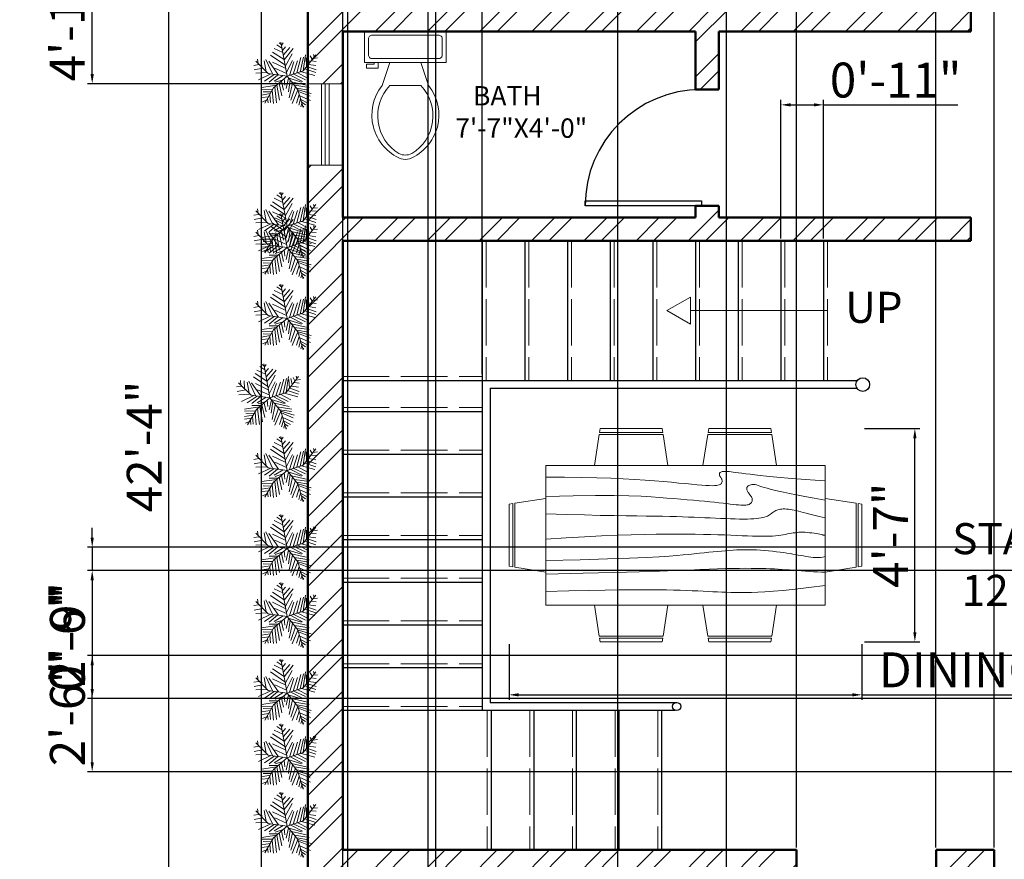
# Model space of a CAD drawing. Units: inches. Extents: x 176 to 806, y 915 to 1663.
# Tile 2 of 5: x 228 to 482, y 1198 to 1414. Entities that reach past the tile are written whole.
import ezdxf

# ---------------------------------------------------------------- set-up
doc = ezdxf.new("R2010")
doc.units = ezdxf.units.IN
doc.linetypes.add('ACAD_ISO02W100', pattern=[15, 12, -3])
for name, color, linetype, lineweight in [('A-ANNO-DIMS', 2, 'Continuous', 18), ('A-ANNO-SYMB', 7, 'Continuous', 18), ('A-ANNO-TEXT', 7, 'Continuous', 18), ('A-AREA-IDEN', 7, 'Continuous', 18), ('A-DOOR', 4, 'Continuous', 25), ('A-FLOR-FIXT', 9, 'Continuous', 18), ('A-FLOR-STRS', 7, 'Continuous', 25), ('A-FLOR-STRS-HIDN', 8, 'ACAD_ISO02W100', 13), ('A-FURN', 8, 'Continuous', 18), ('A-WALL', 7, 'Continuous', 50), ('A-WALL-PATT', 252, 'Continuous', 13), ('C-PROP', 8, 'Continuous', 25), ('L-PLNT', 3, 'Continuous', 13)]:
    doc.layers.add(name, color=color, linetype=linetype, lineweight=lineweight)
doc.layers.add('A-GLAZ', color=244, linetype='Continuous', lineweight=18, true_color=0x991b1e)
doc.styles.get("Standard").update_dxf_attribs({"font": 'arial.ttf'})
doc.dimstyles.new('ISO-25', dxfattribs={"dimtxt": 9, "dimasz": 2.5, "dimexe": 1.25, "dimexo": 0.625, "dimtad": 1, "dimlunit": 3, "dimtxsty": 'Standard', "dimcen": 2.5, "dimadec": 0, "dimazin": 0, "dimtfac": 1, "dimtmove": 0, "dimatfit": 3, "dimfxl": 1, "dimarcsym": 0})

# ---------------------------------------------------------------- blocks, each defined once
blk = doc.blocks.new('*U5')
for p, q in [((0, 0), (0, -6)), ((40, 0), (40, -6))]:
    blk.add_line(p, q)
blk.add_lwpolyline([(0, 0), (0, 40), (1.75, 40), (1.75, 0)], close=True)
blk.add_arc((0, 0), 40, 0, 90)
blk = doc.blocks.new('*D10')
at = {"layer": 'A-ANNO-DIMS', "color": 0, "lineweight": -2, "transparency": 16777216}
for p, q in [((302.08, 1558.21), (265.58, 1558.21)), ((266.83, 1052.71), (266.83, 1555.71)), ((302.08, 1050.21), (265.58, 1050.21))]:
    blk.add_line(p, q, dxfattribs=at)
at = {"layer": 'A-ANNO-DIMS', "color": 0, "transparency": 16777216}
for points in [[(266.42, 1555.71), (267.25, 1555.71), (266.83, 1558.21)], [(266.42, 1052.71), (267.25, 1052.71), (266.83, 1050.21)]]:
    blk.add_solid(points, dxfattribs=at)
at = {"layer": 'Defpoints', "color": 0, "transparency": 16777216}
for p in [(266.83, 1558.21), (302.7, 1558.21), (302.7, 1050.21)]:
    blk.add_point(p, dxfattribs=at)
at = {"layer": 'A-ANNO-DIMS', "color": 0, "transparency": 16777216, "insert": (261.69, 1304.21), "char_height": 9, "attachment_point": 5, "rotation": 90}
blk.add_mtext('42\'-4"', dxfattribs=at)
blk = doc.blocks.new('*U13')
for p, q in [((9.5, -6), (9.5, -2)), ((-10, -8.5), (-8, -8.5)), ((-10, -9.5), (-10, -8.5)), ((-7, -9.5), (-10, -9.5)), ((-8, -8.5), (-8, -8)), ((-7, -8), (-7, -9.5)), ((-4, -8), (-6, -14)), ((4, -8), (6, -14)), ((4, -14), (-4, -14))]:
    blk.add_line(p, q)
blk.add_lwpolyline([(10.5, -8), (10.5, 0), (-10.5, 0), (-10.5, -8)], close=True)
for points in [[(-9.5, -2), (-9.5, -6)], [(8.5, -1), (-8.5, -1)], [(-8.5, -7), (8.5, -7)]]:
    blk.add_lwpolyline(points)
for centre, radius, start, end in [((-8.62, -1.88), 0.884, 81.8699, 188.1301), ((8.62, -1.88), 0.884, 351.8699, 98.1301), ((-8.62, -6.12), 0.884, 171.8699, 278.1301), ((8.62, -6.12), 0.884, 261.8699, 8.1301), ((3.52, -21.58), 12.17, 141.4691, 247.9714), ((4.2, -21.82), 11.33, 136.3677, 238.9468), ((-3.52, -21.58), 12.17, 292.0284, 38.5307), ((-4.2, -21.82), 11.33, 301.053, 43.6321), ((0, -27.88), 4, 245.7318, 294.2682), ((0, -29), 4, 254.8605, 285.1395)]:
    blk.add_arc(centre, radius, start, end)
blk = doc.blocks.new('Dining Set - 36 x 72 in.')
for p, q in [((-22.2343, 26.00059), (-23.4847, 17.99762)), ((-22.2304, 26), (-5.7608, 26)), ((-22, 27.5), (-22.1562, 26.50042)), ((-5.8416, 26.5), (-22.1534, 26.5)), ((-22, 27.5), (-6, 27.5)), ((-5.8437, 26.49966), (-6, 27.5)), ((-4.5152, 17.99762), (-5.7655, 25.99926)), ((5.7657, 26.00059), (4.5153, 17.99762)), ((5.7696, 26), (22.2392, 26)), ((6, 27.5), (5.8438, 26.50042)), ((22.1584, 26.5), (5.8466, 26.5)), ((6, 27.5), (22, 27.5)), ((22.1563, 26.49966), (22, 27.5)), ((23.4848, 17.99762), (22.2345, 25.99926)), ((36, 18), (-36, 18)), ((-36, 18), (-36, -18)), ((36, -18), (36, 18)), ((-45.5, 8), (-44.5004, 8.15617)), ((-45.5, 8), (-45.5, -8)), ((-44.5, -8.15843), (-44.5, 8.15338)), ((-44.0006, 8.23428), (-35.9976, 9.48474)), ((-44, 8.23041), (-44, -8.23915)), ((44.0006, 8.23428), (35.9976, 9.48474)), ((44, 8.23041), (44, -8.23915)), ((44.5, -8.15843), (44.5, 8.15338)), ((45.5, 8), (44.5005, 8.15617)), ((45.5, 8), (45.5, -8)), ((-44.4997, -8.15631), (-45.5, -8)), ((-35.9976, -9.48476), (-43.9993, -8.2345)), ((35.9976, -9.48476), (43.9993, -8.2345)), ((44.4997, -8.15631), (45.5, -8)), ((-36, -18), (36, -18)), ((-22.2343, -26.0006), (-23.4847, -17.99762)), ((-4.5152, -17.99762), (-5.7655, -25.99928)), ((5.7657, -26.0006), (4.5153, -17.99762)), ((23.4848, -17.99762), (22.2345, -25.99928)), ((-22.2304, -26), (-5.7608, -26)), ((-22, -27.5), (-22.1562, -26.50044)), ((-5.8416, -26.5), (-22.1534, -26.5)), ((-22, -27.5), (-6, -27.5)), ((-5.8437, -26.49967), (-6, -27.5)), ((5.7696, -26), (22.2392, -26)), ((6, -27.5), (5.8438, -26.50044)), ((22.1584, -26.5), (5.8466, -26.5)), ((6, -27.5), (22, -27.5)), ((22.1563, -26.49967), (22, -27.5))]:
    blk.add_line(p, q)
for points in [[(-36, 15), (-31.1772, 14.97754), (-26.8079, 14.91406), (-22.8538, 14.81543), (-19.276, 14.6875), (-16.0362, 14.53613), (-13.0957, 14.36718), (-10.4159, 14.18652), (-7.9583, 14), (-5.6904, 13.81315), (-3.6035, 13.63021), (-1.6954, 13.45508), (0.0365, 13.29166), (1.5945, 13.14388), (2.9811, 13.01562), (4.1988, 12.9108), (5.25, 12.83333), (6.1393, 12.78613), (6.8802, 12.76823), (7.4883, 12.77767), (7.9792, 12.8125), (8.3685, 12.87077), (8.6719, 12.95052), (8.9049, 13.0498), (9.0833, 13.16666), (9.2205, 13.29899), (9.3216, 13.44401), (9.3895, 13.59879), (9.4271, 13.76041), (9.4373, 13.92594), (9.4232, 14.09245), (9.3875, 14.257), (9.3333, 14.41666), (9.2638, 14.56917), (9.1836, 14.71484), (9.0975, 14.85465), (9.0104, 14.98958), (8.9272, 15.1206), (8.8529, 15.2487), (8.7922, 15.37483), (8.75, 15.5), (8.7305, 15.62467), (8.7344, 15.74739), (8.7617, 15.86621), (8.8125, 15.97916), (8.8867, 16.08431), (8.9844, 16.17968), (9.1055, 16.26334), (9.25, 16.33333), (9.4189, 16.38802), (9.6172, 16.42708), (9.8506, 16.45052), (10.125, 16.45833), (10.4463, 16.45052), (10.8203, 16.42708), (11.2529, 16.38802), (11.75, 16.33333), (12.3184, 16.26318), (12.9694, 16.17838), (13.7151, 16.07991), (14.5677, 15.96875), (15.5395, 15.84586), (16.6426, 15.71224), (17.8893, 15.56884), (19.2917, 15.41666), (20.859, 15.25667), (22.5879, 15.08984), (24.4721, 14.91715), (26.5052, 14.73958), (28.6809, 14.5581), (30.9929, 14.3737), (33.4347, 14.18733), (36, 14)], [(-36, 10), (-28.9766, 10.14274), (-23.1725, 10.20442), (-18.4241, 10.19775), (-14.5677, 10.13541), (-11.4399, 10.03011), (-8.877, 9.89453), (-6.7154, 9.74137), (-4.7917, 9.58333), (-2.9698, 9.43082), (-1.2246, 9.28515), (0.4415, 9.14534), (2.026, 9.01041), (3.5266, 8.87939), (4.9408, 8.7513), (6.266, 8.62516), (7.5, 8.5), (8.6411, 8.37549), (9.6914, 8.2539), (10.6538, 8.13818), (11.5312, 8.03125), (12.3267, 7.93603), (13.043, 7.85547), (13.6831, 7.79248), (14.25, 7.75), (14.7471, 7.7303), (15.1797, 7.73307), (15.5537, 7.75732), (15.875, 7.80208), (16.1494, 7.86637), (16.3828, 7.94922), (16.5811, 8.04964), (16.75, 8.16666), (16.8944, 8.29915), (17.0143, 8.44531), (17.1089, 8.60319), (17.1771, 8.77083), (17.218, 8.94629), (17.2305, 9.1276), (17.2137, 9.31282), (17.1667, 9.5), (17.0895, 9.6875), (16.987, 9.875), (16.8649, 10.0625), (16.7292, 10.25), (16.5856, 10.4375), (16.4401, 10.625), (16.2985, 10.8125), (16.1667, 11), (16.05, 11.18733), (15.9518, 11.3737), (15.8752, 11.5581), (15.8229, 11.73958), (15.798, 11.91715), (15.8034, 12.08984), (15.842, 12.25667), (15.9167, 12.41666), (16.0295, 12.56836), (16.1784, 12.70833), (16.3605, 12.83268), (16.5729, 12.9375), (16.8127, 13.01888), (17.0768, 13.07291), (17.3625, 13.0957), (17.6667, 13.08333), (17.9894, 13.03312), (18.3418, 12.94726), (18.7382, 12.82918), (19.1927, 12.68229), (19.7195, 12.51001), (20.3327, 12.31575), (21.0465, 12.10294), (21.875, 11.875), (22.8357, 11.63354), (23.959, 11.37304), (25.2786, 11.08618), (26.8282, 10.76562), (28.6414, 10.40405), (30.752, 9.99414), (33.1936, 9.52856), (36, 9)], [(-36, 5.5), (-30.7157, 5.3348), (-26.069, 5.20963), (-21.9946, 5.11767), (-18.4271, 5.05208), (-15.3009, 5.00602), (-12.5508, 4.97265), (-10.1112, 4.94515), (-7.9167, 4.91666), (-5.909, 4.88167), (-4.0586, 4.83984), (-2.3429, 4.79215), (-0.7396, 4.73958), (0.7739, 4.6831), (2.22, 4.6237), (3.6213, 4.56233), (5, 4.5), (6.373, 4.43782), (7.7344, 4.3776), (9.0723, 4.32129), (10.375, 4.27083), (11.6309, 4.22819), (12.8281, 4.19531), (13.9551, 4.17415), (15, 4.16666), (15.954, 4.17448), (16.819, 4.19791), (17.6001, 4.23698), (18.3021, 4.29166), (18.9299, 4.36198), (19.4883, 4.44791), (19.9823, 4.54948), (20.4167, 4.66666), (20.7969, 4.79899), (21.1302, 4.94401), (21.4245, 5.09879), (21.6875, 5.26041), (21.9271, 5.42594), (22.1511, 5.59245), (22.3672, 5.757), (22.5834, 5.91666), (22.8065, 6.06868), (23.0404, 6.21093), (23.2879, 6.34147), (23.5521, 6.45833), (23.8358, 6.55957), (24.142, 6.64323), (24.4735, 6.70735), (24.8334, 6.75), (25.2235, 6.76969), (25.642, 6.76692), (26.0858, 6.74267), (26.5521, 6.69791), (27.0379, 6.63362), (27.5404, 6.55078), (28.0565, 6.45036), (28.5834, 6.33333), (29.1242, 6.19987), (29.7071, 6.04687), (30.3661, 5.87044), (31.1354, 5.66666), (32.0493, 5.43164), (33.142, 5.16146), (34.4475, 4.85221), (36, 4.5)], [(-36, -1), (-30.7915, -0.6591), (-26.0195, -0.38216), (-21.6519, -0.16284), (-17.6563, 0.00521), (-14.0005, 0.12833), (-10.6523, 0.21289), (-7.5796, 0.26522), (-4.75, 0.29166), (-2.134, 0.29793), (0.2878, 0.28711), (2.5317, 0.26163), (4.6146, 0.22396), (6.5529, 0.17651), (8.3633, 0.12174), (10.0623, 0.06209), (11.6667, 0), (13.1899, -0.06201), (14.6341, -0.1211), (15.9982, -0.17432), (17.2813, -0.21875), (18.4823, -0.25147), (19.6003, -0.26953), (20.6343, -0.27002), (21.5834, -0.25), (22.4481, -0.20768), (23.2357, -0.14584), (23.9549, -0.06836), (24.6146, 0.02083), (25.2235, 0.11784), (25.7904, 0.21875), (26.3241, 0.31966), (26.8334, 0.41666), (27.3265, 0.50618), (27.8099, 0.58593), (28.2894, 0.65397), (28.7709, 0.70833), (29.2601, 0.74707), (29.763, 0.76823), (30.2855, 0.76985), (30.8334, 0.75), (31.4088, 0.70784), (31.9994, 0.64713), (32.589, 0.57275), (33.1615, 0.48958), (33.7008, 0.4025), (34.1908, 0.3164), (34.6153, 0.23616), (34.9584, 0.16666), (35.2099, 0.11165), (35.3848, 0.07031), (35.504, 0.04069), (35.5886, 0.02083), (35.6594, 0.00879), (35.7377, 0.0026), (35.8442, 0.00032), (36, 0)], [(-36, -6.5), (-27.1843, -6.31267), (-20.084, -6.1263), (-14.469, -5.9419), (-10.1094, -5.76042), (-6.7752, -5.58285), (-4.2363, -5.41016), (-2.2629, -5.24333), (-0.625, -5.08334), (0.8708, -4.93099), (2.2715, -4.78646), (3.5872, -4.64974), (4.8281, -4.52084), (6.0046, -4.39974), (7.127, -4.28646), (8.2053, -4.18099), (9.25, -4.08334), (10.2705, -3.99382), (11.2734, -3.91407), (12.2647, -3.84603), (13.25, -3.79167), (14.2354, -3.75293), (15.2266, -3.73177), (16.2295, -3.73015), (17.25, -3.75), (18.2912, -3.79248), (19.3451, -3.85547), (20.4009, -3.93604), (21.4479, -4.03125), (22.4754, -4.13819), (23.4727, -4.25391), (24.4289, -4.37549), (25.3334, -4.5), (26.1785, -4.62492), (26.9694, -4.74935), (27.7145, -4.87281), (28.4219, -4.99479), (29.1, -5.11483), (29.7572, -5.23242), (30.4016, -5.34709), (31.0417, -5.45834), (31.6837, -5.56437), (32.3262, -5.65821), (32.9658, -5.73153), (33.599, -5.77604), (34.2224, -5.78345), (34.8327, -5.74545), (35.4264, -5.65373), (36, -5.5)], [(-36, -10), (-26.4022, -9.81299), (-18.4675, -9.62891), (-11.9839, -9.45069), (-6.7396, -9.28125), (-2.5226, -9.12354), (0.8789, -8.98047), (3.6769, -8.85498), (6.0833, -8.75), (8.2767, -8.66765), (10.3021, -8.60677), (12.1712, -8.56543), (13.8958, -8.54167), (15.4876, -8.53353), (16.9583, -8.53907), (18.3197, -8.55632), (19.5834, -8.58334), (20.7616, -8.61841), (21.8685, -8.66081), (22.9188, -8.71004), (23.9271, -8.76563), (24.9081, -8.82707), (25.8763, -8.89388), (26.8465, -8.96558), (27.8334, -9.04167), (28.8474, -9.12118), (29.8828, -9.20117), (30.93, -9.27824), (31.9792, -9.34896), (33.0205, -9.40991), (34.0443, -9.45768), (35.0407, -9.48885), (36, -9.5)], [(-36, -14.5), (-30.0881, -14.33513), (-25.0332, -14.21224), (-20.7312, -14.12647), (-17.0781, -14.07292), (-13.97, -14.04671), (-11.3027, -14.04297), (-8.9724, -14.05681), (-6.875, -14.08334), (-4.9224, -14.11833), (-3.0905, -14.16016), (-1.3709, -14.20785), (0.2448, -14.26042), (1.7647, -14.3169), (3.1973, -14.3763), (4.5507, -14.43767), (5.8333, -14.5), (7.0554, -14.5621), (8.235, -14.62175), (9.3922, -14.67652), (10.5469, -14.72396), (11.7192, -14.76164), (12.929, -14.78711), (14.1965, -14.79794), (15.5417, -14.79167), (16.9933, -14.76424), (18.6152, -14.70508), (20.4804, -14.60197), (22.6615, -14.44271), (25.2312, -14.21509), (28.2624, -13.9069), (31.8277, -13.50594), (36, -13)]]:
    blk.add_lwpolyline(points)
blk = doc.blocks.new('*U8')
for p, q in [((-8.737, 47.138), (-17.069, 52.711)), ((-10.186, 53.64), (-13.084, 55.962)), ((0, 0), (-10.5, 57)), ((-9.099, 51.782), (-6.563, 55.962)), ((-3.665, 19.273), (-27.574, 35.527)), ((-5.114, 28.097), (-24.676, 40.636)), ((-7.288, 39.707), (-21.778, 46.673)), ((-7.65, 43.423), (-2.578, 49.46)), ((-5.839, 35.992), (4.667, 48.067)), ((-5.114, 27.632), (10.463, 46.673)), ((-2.941, 16.486), (8.652, 37.85)), ((27, 9), (48, 36)), ((27.127, 9.056), (31.112, 35.992)), ((38.719, 34.134), (41.979, 28.561)), ((44.153, 36.456), (45.239, 32.741)), ((-47.498, 19.737), (-55.83, 18.344)), ((-31.5, 4.5), (-52.5, 25.5)), ((-48.585, 21.131), (-49.309, 29.026)), ((-43.513, 28.561), (-42.427, 15.558)), ((-38.442, 26.239), (-34.819, 7.663)), ((-35.544, 28.097), (-24.314, 3.947)), ((-14.533, 2.09), (-30.834, 25.31)), ((-24.314, 23.917), (-2.941, 13.7)), ((-1.129, 6.734), (9.014, 26.704)), ((3.942, 1.625), (11.187, 24.381)), ((10.101, 3.483), (17.708, 26.239)), ((16.259, 5.805), (23.142, 31.348)), ((22.055, 7.198), (27.489, 32.277)), ((31.836, 30.883), (32.561, 16.486)), ((35.096, 32.741), (37.27, 22.524)), ((36.183, 19.737), (48.137, 17.88)), ((40.53, 25.775), (48.862, 24.846)), ((43.791, 29.954), (51.036, 30.883)), ((-40.615, 13.7), (-55.105, 10.913)), ((-33.37, 6.269), (-52.207, 5.34)), ((-28.299, 3.483), (-47.86, -5.805)), ((-21.416, 3.018), (-38.079, -8.128)), ((0, 0), (-31.5, 4.5)), ((-15.982, 2.09), (-30.11, -9.521)), ((0, 0), (-22.5, -19.5)), ((-6.563, 1.161), (-21.416, -8.128)), ((-20.691, 13.7), (-1.129, 4.876)), ((0, 0), (27, 9)), ((0, 0), (18, -22.5)), ((6.478, 1.625), (26.04, -8.592)), ((11.187, 3.483), (30.749, -5.805)), ((18.07, 5.805), (35.096, -3.483)), ((24.229, 7.663), (46.688, 1.625)), ((29.662, 12.307), (48.137, 6.269)), ((33.285, 16.486), (48.862, 10.913)), ((-17.431, -15.094), (-42.789, -18.809)), ((-15.257, -12.772), (-30.11, -12.772)), ((-6.563, -5.805), (-19.967, -9.985)), ((-17.069, -15.094), (-12.721, -40.172)), ((-13.446, -11.378), (-8.737, -32.741)), ((-9.461, -8.592), (-6.201, -23.453)), ((-4.752, -3.483), (-3.665, -14.629)), ((2.493, -3.019), (-1.491, -20.202)), ((1.769, -2.555), (24.229, -9.521)), ((5.029, -6.27), (2.131, -25.775)), ((9.014, -11.378), (3.58, -35.992)), ((7.565, -9.056), (32.198, -14.629)), ((12.274, -15.094), (36.907, -18.809)), ((-28.299, -29.026), (-42.789, -31.348)), ((-24.314, -21.596), (-42.427, -22.06)), ((-26.849, -26.24), (-40.253, -25.775)), ((-22.5, -19.5), (-37.5, -45)), ((-29.023, -30.884), (-27.936, -43.887)), ((-25.038, -23.918), (-22.865, -45.281)), ((-20.691, -18.345), (-17.793, -44.352)), ((14.085, -16.951), (6.478, -40.172)), ((18.07, -22.524), (8.289, -45.745)), ((20.244, -30.419), (15.897, -44.816)), ((16.259, -19.738), (36.183, -22.989)), ((18, -22.5), (27, -52.5)), ((18.433, -22.524), (40.53, -29.026)), ((19.157, -25.311), (38.719, -33.206)), ((21.331, -32.741), (39.081, -40.636)), ((-30.834, -34.135), (-42.427, -35.528)), ((-34.457, -39.708), (-40.978, -42.494)), ((-32.646, -36.921), (-31.921, -44.352)), ((22.78, -37.85), (19.519, -48.532)), ((22.78, -38.314), (34.372, -44.816)), ((24.591, -45.745), (23.142, -50.854)), ((24.591, -43.423), (30.749, -47.603)), ((26.764, -49.925), (28.213, -50.854))]:
    blk.add_line(p, q)
blk = doc.blocks.new('WIN-GLAZING-21IN')
for p, q in [((0, 1), (21, 1)), ((0, 0), (21, 0)), ((0, -1), (21, -1))]:
    blk.add_line(p, q)
blk = doc.blocks.new('*D34')
at = {"layer": 'A-ANNO-DIMS', "color": 0, "lineweight": -2, "transparency": 16777216}
for p, q in [((354.6, 1253.2), (354.6, 1238.92)), ((445.6, 1253.2), (445.6, 1238.92)), ((357.1, 1240.17), (443.1, 1240.17)), ((445.6, 1240.17), (548.27, 1240.17))]:
    blk.add_line(p, q, dxfattribs=at)
at = {"layer": 'A-ANNO-DIMS', "color": 0, "transparency": 16777216}
for points in [[(357.1, 1240.59), (357.1, 1239.75), (354.6, 1240.17)], [(443.1, 1240.59), (443.1, 1239.75), (445.6, 1240.17)]]:
    blk.add_solid(points, dxfattribs=at)
at = {"layer": 'Defpoints', "color": 0, "transparency": 16777216}
for p in [(354.6, 1253.82), (445.6, 1253.82), (445.6, 1240.17)]:
    blk.add_point(p, dxfattribs=at)
at = {"layer": 'A-ANNO-DIMS', "color": 0, "transparency": 16777216, "insert": (498.18, 1245.45), "char_height": 9, "attachment_point": 5}
blk.add_mtext('DINING SET 7\'-7"', dxfattribs=at)
blk = doc.blocks.new('*D35')
at = {"layer": 'A-ANNO-DIMS', "color": 0, "lineweight": -2, "transparency": 16777216}
for p, q in [((446.22, 1308.82), (460.5, 1308.82)), ((459.25, 1256.32), (459.25, 1306.32)), ((446.22, 1253.82), (460.5, 1253.82))]:
    blk.add_line(p, q, dxfattribs=at)
at = {"layer": 'A-ANNO-DIMS', "color": 0, "transparency": 16777216}
for points in [[(458.83, 1306.32), (459.66, 1306.32), (459.25, 1308.82)], [(458.83, 1256.32), (459.66, 1256.32), (459.25, 1253.82)]]:
    blk.add_solid(points, dxfattribs=at)
at = {"layer": 'Defpoints', "color": 0, "transparency": 16777216}
for p in [(445.6, 1308.82), (459.25, 1308.82), (445.6, 1253.82)]:
    blk.add_point(p, dxfattribs=at)
at = {"layer": 'A-ANNO-DIMS', "color": 0, "transparency": 16777216, "insert": (454.12, 1281.32), "char_height": 9, "attachment_point": 5, "rotation": 90}
blk.add_mtext('4\'-7"', dxfattribs=at)
blk = doc.blocks.new('*D48')
at = {"layer": 'A-ANNO-DIMS', "color": 0, "lineweight": -2, "transparency": 16777216}
for p, q in [((302.08, 1447.21), (245.85, 1447.21)), ((247.1, 1400.21), (247.1, 1444.71)), ((302.08, 1397.71), (245.85, 1397.71))]:
    blk.add_line(p, q, dxfattribs=at)
at = {"layer": 'A-ANNO-DIMS', "color": 0, "transparency": 16777216}
for points in [[(246.68, 1444.71), (247.52, 1444.71), (247.1, 1447.21)], [(246.68, 1400.21), (247.52, 1400.21), (247.1, 1397.71)]]:
    blk.add_solid(points, dxfattribs=at)
at = {"layer": 'Defpoints', "color": 0, "transparency": 16777216}
for p in [(247.1, 1447.21), (302.7, 1447.21), (302.7, 1397.71)]:
    blk.add_point(p, dxfattribs=at)
at = {"layer": 'A-ANNO-DIMS', "color": 0, "transparency": 16777216, "insert": (241.82, 1422.46), "char_height": 9, "attachment_point": 5, "rotation": 90}
blk.add_mtext('4\'-1 1/2"', dxfattribs=at)
blk = doc.blocks.new('*D50')
at = {"layer": 'A-ANNO-DIMS', "color": 0, "lineweight": -2, "transparency": 16777216}
for p, q in [((311.7, 1321.83), (311.7, 1645.51)), ((347.7, 1322.83), (347.7, 1645.51)), ((314.2, 1644.26), (345.2, 1644.26))]:
    blk.add_line(p, q, dxfattribs=at)
at = {"layer": 'A-ANNO-DIMS', "color": 0, "transparency": 16777216}
for points in [[(314.2, 1644.67), (314.2, 1643.84), (311.7, 1644.26)], [(345.2, 1644.67), (345.2, 1643.84), (347.7, 1644.26)]]:
    blk.add_solid(points, dxfattribs=at)
at = {"layer": 'Defpoints', "color": 0, "transparency": 16777216}
for p in [(347.7, 1644.26), (311.7, 1321.21), (347.7, 1322.21)]:
    blk.add_point(p, dxfattribs=at)
at = {"layer": 'A-ANNO-DIMS', "color": 0, "transparency": 16777216, "insert": (329.7, 1649.48), "char_height": 9, "attachment_point": 5}
blk.add_mtext('3\'-0"', dxfattribs=at)
blk = doc.blocks.new('*D52')
at = {"layer": 'A-ANNO-DIMS', "color": 0, "lineweight": -2, "transparency": 16777216}
for p, q in [((479.7, 1200.83), (479.7, 1645.51)), ((527.7, 1200.83), (527.7, 1645.51)), ((482.2, 1644.26), (525.2, 1644.26))]:
    blk.add_line(p, q, dxfattribs=at)
at = {"layer": 'A-ANNO-DIMS', "color": 0, "transparency": 16777216}
for points in [[(482.2, 1644.67), (482.2, 1643.84), (479.7, 1644.26)], [(525.2, 1644.67), (525.2, 1643.84), (527.7, 1644.26)]]:
    blk.add_solid(points, dxfattribs=at)
at = {"layer": 'Defpoints', "color": 0, "transparency": 16777216}
for p in [(527.7, 1644.26), (479.7, 1200.21), (527.7, 1200.21)]:
    blk.add_point(p, dxfattribs=at)
at = {"layer": 'A-ANNO-DIMS', "color": 0, "transparency": 16777216, "insert": (503.7, 1649.48), "char_height": 9, "attachment_point": 5}
blk.add_mtext('4\'-0"', dxfattribs=at)
blk = doc.blocks.new('*D54')
at = {"layer": 'A-ANNO-DIMS', "color": 0, "lineweight": -2, "transparency": 16777216}
for p, q in [((247.1, 1280.71), (247.1, 1283.21)), ((614.08, 1278.21), (245.85, 1278.21)), ((247.1, 1278.21), (247.1, 1272.21)), ((614.08, 1272.21), (245.85, 1272.21)), ((247.1, 1269.71), (247.1, 1242.03))]:
    blk.add_line(p, q, dxfattribs=at)
at = {"layer": 'A-ANNO-DIMS', "color": 0, "transparency": 16777216}
for points in [[(246.68, 1280.71), (247.52, 1280.71), (247.1, 1278.21)], [(246.68, 1269.71), (247.52, 1269.71), (247.1, 1272.21)]]:
    blk.add_solid(points, dxfattribs=at)
at = {"layer": 'Defpoints', "color": 0, "transparency": 16777216}
for p in [(614.7, 1278.21), (247.1, 1272.21), (614.7, 1272.21)]:
    blk.add_point(p, dxfattribs=at)
at = {"layer": 'A-ANNO-DIMS', "color": 0, "transparency": 16777216, "insert": (241.88, 1254.62), "char_height": 9, "attachment_point": 5, "rotation": 90}
blk.add_mtext('0\'-6"', dxfattribs=at)
blk = doc.blocks.new('*D57')
at = {"layer": 'A-ANNO-DIMS', "color": 0, "lineweight": -2, "transparency": 16777216}
for p, q in [((382.69, 1071.94), (382.69, 1645.51)), ((410.64, 1071.94), (410.64, 1645.51)), ((385.19, 1644.26), (408.14, 1644.26))]:
    blk.add_line(p, q, dxfattribs=at)
at = {"layer": 'A-ANNO-DIMS', "color": 0, "transparency": 16777216}
for points in [[(385.19, 1644.67), (385.19, 1643.84), (382.69, 1644.26)], [(408.14, 1644.67), (408.14, 1643.84), (410.64, 1644.26)]]:
    blk.add_solid(points, dxfattribs=at)
at = {"layer": 'Defpoints', "color": 0, "transparency": 16777216}
for p in [(410.64, 1644.26), (382.69, 1071.32), (410.64, 1071.32)]:
    blk.add_point(p, dxfattribs=at)
at = {"layer": 'A-ANNO-DIMS', "color": 0, "transparency": 16777216, "insert": (396.67, 1649.4), "char_height": 9, "attachment_point": 5}
blk.add_mtext('2\'-4"', dxfattribs=at)
blk = doc.blocks.new('*D58')
at = {"layer": 'A-ANNO-DIMS', "color": 0, "lineweight": -2, "transparency": 16777216}
for p, q in [((654.08, 1250.31), (245.85, 1250.31)), ((247.1, 1222.81), (247.1, 1247.81)), ((654.08, 1220.31), (245.85, 1220.31))]:
    blk.add_line(p, q, dxfattribs=at)
at = {"layer": 'A-ANNO-DIMS', "color": 0, "transparency": 16777216}
for points in [[(246.68, 1247.81), (247.52, 1247.81), (247.1, 1250.31)], [(246.68, 1222.81), (247.52, 1222.81), (247.1, 1220.31)]]:
    blk.add_solid(points, dxfattribs=at)
at = {"layer": 'Defpoints', "color": 0, "transparency": 16777216}
for p in [(247.1, 1250.31), (654.7, 1250.31), (654.7, 1220.31)]:
    blk.add_point(p, dxfattribs=at)
at = {"layer": 'A-ANNO-DIMS', "color": 0, "transparency": 16777216, "insert": (241.88, 1235.31), "char_height": 9, "attachment_point": 5, "rotation": 90}
blk.add_mtext('2\'-6"', dxfattribs=at)
blk = doc.blocks.new('*D59')
at = {"layer": 'A-ANNO-DIMS', "color": 0, "lineweight": -2, "transparency": 16777216}
for p, q in [((428.7, 1200.83), (428.7, 1645.51)), ((464.7, 1200.83), (464.7, 1645.51)), ((431.2, 1644.26), (462.2, 1644.26))]:
    blk.add_line(p, q, dxfattribs=at)
at = {"layer": 'A-ANNO-DIMS', "color": 0, "transparency": 16777216}
for points in [[(431.2, 1644.67), (431.2, 1643.84), (428.7, 1644.26)], [(462.2, 1644.67), (462.2, 1643.84), (464.7, 1644.26)]]:
    blk.add_solid(points, dxfattribs=at)
at = {"layer": 'Defpoints', "color": 0, "transparency": 16777216}
for p in [(464.7, 1644.26), (428.7, 1200.21), (464.7, 1200.21)]:
    blk.add_point(p, dxfattribs=at)
at = {"layer": 'A-ANNO-DIMS', "color": 0, "transparency": 16777216, "insert": (446.7, 1649.48), "char_height": 9, "attachment_point": 5}
blk.add_mtext('3\'-0"', dxfattribs=at)
blk = doc.blocks.new('*D61')
at = {"layer": 'A-ANNO-DIMS', "color": 0, "lineweight": -2, "transparency": 16777216}
for p, q in [((311.7, 1191.83), (311.7, 1645.51)), ((335.7, 1191.83), (335.7, 1645.51)), ((314.2, 1644.26), (333.2, 1644.26)), ((335.7, 1644.26), (363.53, 1644.26))]:
    blk.add_line(p, q, dxfattribs=at)
at = {"layer": 'A-ANNO-DIMS', "color": 0, "transparency": 16777216}
for points in [[(314.2, 1644.67), (314.2, 1643.84), (311.7, 1644.26)], [(333.2, 1644.67), (333.2, 1643.84), (335.7, 1644.26)]]:
    blk.add_solid(points, dxfattribs=at)
at = {"layer": 'Defpoints', "color": 0, "transparency": 16777216}
for p in [(335.7, 1644.26), (311.7, 1191.21), (335.7, 1191.21)]:
    blk.add_point(p, dxfattribs=at)
at = {"layer": 'A-ANNO-DIMS', "color": 0, "transparency": 16777216, "insert": (350.87, 1649.48), "char_height": 9, "attachment_point": 5}
blk.add_mtext('2\'-0"', dxfattribs=at)
blk = doc.blocks.new('*D62')
at = {"layer": 'A-ANNO-DIMS', "color": 0, "lineweight": -2, "transparency": 16777216}
for p, q in [((313.06, 1169.74), (313.06, 1645.51)), ((333.74, 1169.74), (333.74, 1645.51)), ((315.56, 1644.26), (331.24, 1644.26)), ((333.74, 1644.26), (381.54, 1644.26))]:
    blk.add_line(p, q, dxfattribs=at)
at = {"layer": 'A-ANNO-DIMS', "color": 0, "transparency": 16777216}
for points in [[(315.56, 1644.67), (315.56, 1643.84), (313.06, 1644.26)], [(331.24, 1644.67), (331.24, 1643.84), (333.74, 1644.26)]]:
    blk.add_solid(points, dxfattribs=at)
at = {"layer": 'Defpoints', "color": 0, "transparency": 16777216}
for p in [(333.74, 1644.26), (313.06, 1169.12), (333.74, 1169.12)]:
    blk.add_point(p, dxfattribs=at)
at = {"layer": 'A-ANNO-DIMS', "color": 0, "transparency": 16777216, "insert": (358.89, 1649.53), "char_height": 9, "attachment_point": 5}
blk.add_mtext('1\'-8 1/2"', dxfattribs=at)
blk = doc.blocks.new('*D63')
at = {"layer": 'A-ANNO-DIMS', "color": 0, "lineweight": -2, "transparency": 16777216}
for p, q in [((783.85, 1169.12), (783.85, 1217.75)), ((334.37, 1169.12), (785.1, 1169.12)), ((783.85, 1129.89), (783.85, 1166.62)), ((334.37, 1127.39), (785.1, 1127.39))]:
    blk.add_line(p, q, dxfattribs=at)
at = {"layer": 'A-ANNO-DIMS', "color": 0, "transparency": 16777216}
for points in [[(783.43, 1166.62), (784.27, 1166.62), (783.85, 1169.12)], [(783.43, 1129.89), (784.27, 1129.89), (783.85, 1127.39)]]:
    blk.add_solid(points, dxfattribs=at)
at = {"layer": 'Defpoints', "color": 0, "transparency": 16777216}
for p in [(333.74, 1169.12), (783.85, 1169.12), (333.74, 1127.39)]:
    blk.add_point(p, dxfattribs=at)
at = {"layer": 'A-ANNO-DIMS', "color": 0, "transparency": 16777216, "insert": (778.57, 1194.68), "char_height": 9, "attachment_point": 5, "rotation": 90}
blk.add_mtext('3\'-5 1/2"', dxfattribs=at)
blk = doc.blocks.new('*D67')
at = {"layer": 'A-ANNO-DIMS', "color": 0, "lineweight": -2, "transparency": 16777216}
for p, q in [((783.85, 1191.21), (783.85, 1225.03)), ((336.33, 1191.21), (785.1, 1191.21)), ((783.85, 1171.62), (783.85, 1188.71)), ((334.37, 1169.12), (785.1, 1169.12))]:
    blk.add_line(p, q, dxfattribs=at)
at = {"layer": 'A-ANNO-DIMS', "color": 0, "transparency": 16777216}
for points in [[(783.43, 1188.71), (784.27, 1188.71), (783.85, 1191.21)], [(783.43, 1171.62), (784.27, 1171.62), (783.85, 1169.12)]]:
    blk.add_solid(points, dxfattribs=at)
at = {"layer": 'Defpoints', "color": 0, "transparency": 16777216}
for p in [(335.7, 1191.21), (783.85, 1191.21), (333.74, 1169.12)]:
    blk.add_point(p, dxfattribs=at)
at = {"layer": 'A-ANNO-DIMS', "color": 0, "transparency": 16777216, "insert": (778.63, 1209.37), "char_height": 9, "attachment_point": 5, "rotation": 90}
blk.add_mtext('1\'-10"', dxfattribs=at)
blk = doc.blocks.new('*D71')
at = {"layer": 'A-ANNO-DIMS', "color": 0, "lineweight": -2, "transparency": 16777216}
for p, q in [((715.11, 1272.21), (245.85, 1272.21)), ((247.1, 1269.71), (247.1, 1241.71)), ((704.61, 1239.21), (245.85, 1239.21))]:
    blk.add_line(p, q, dxfattribs=at)
at = {"layer": 'A-ANNO-DIMS', "color": 0, "transparency": 16777216}
for points in [[(246.68, 1269.71), (247.52, 1269.71), (247.1, 1272.21)], [(246.68, 1241.71), (247.52, 1241.71), (247.1, 1239.21)]]:
    blk.add_solid(points, dxfattribs=at)
at = {"layer": 'Defpoints', "color": 0, "transparency": 16777216}
for p in [(715.73, 1272.21), (247.1, 1239.21), (705.23, 1239.21)]:
    blk.add_point(p, dxfattribs=at)
at = {"layer": 'A-ANNO-DIMS', "color": 0, "transparency": 16777216, "insert": (241.88, 1255.71), "char_height": 9, "attachment_point": 5, "rotation": 90}
blk.add_mtext('2\'-9"', dxfattribs=at)
blk = doc.blocks.new('*D72')
at = {"layer": 'A-ANNO-DIMS', "color": 0, "lineweight": -2, "transparency": 16777216}
for p, q in [((424.7, 1357.83), (424.7, 1393.51)), ((427.2, 1392.26), (433.2, 1392.26)), ((435.7, 1357.83), (435.7, 1393.51)), ((435.7, 1392.26), (470.37, 1392.26))]:
    blk.add_line(p, q, dxfattribs=at)
at = {"layer": 'A-ANNO-DIMS', "color": 0, "transparency": 16777216}
for points in [[(427.2, 1392.67), (427.2, 1391.84), (424.7, 1392.26)], [(433.2, 1392.67), (433.2, 1391.84), (435.7, 1392.26)]]:
    blk.add_solid(points, dxfattribs=at)
at = {"layer": 'Defpoints', "color": 0, "transparency": 16777216}
for p in [(435.7, 1392.26), (424.7, 1357.21), (435.7, 1357.21)]:
    blk.add_point(p, dxfattribs=at)
at = {"layer": 'A-ANNO-DIMS', "color": 0, "transparency": 16777216, "insert": (454.29, 1397.48), "char_height": 9, "attachment_point": 5}
blk.add_mtext('0\'-11"', dxfattribs=at)

msp = doc.modelspace()

# ---------------------------------------------------------------- hatches: boundary and pattern name
at = {"layer": 'A-WALL-PATT'}
h = msp.add_hatch(dxfattribs=at)
h.set_pattern_fill('ANSI32', color=256)
h.paths.add_polyline_path([(302.704, 1050.206), (353.704, 1050.206), (353.704, 1059.206), (311.704, 1059.206), (311.704, 1191.206), (428.704, 1191.206), (428.704, 1200.206), (311.704, 1200.206), (311.704, 1357.206), (473.704, 1357.206), (473.704, 1363.206), (408.704, 1363.206), (408.704, 1366.206), (402.704, 1366.206), (402.704, 1363.206), (311.704, 1363.206), (311.704, 1376.706), (302.704, 1376.706)])
h.paths.add_polyline_path([(311.704, 1447.206), (302.704, 1447.206), (302.704, 1397.706), (311.704, 1397.706), (311.704, 1411.206), (402.704, 1411.206), (402.704, 1396.206), (408.704, 1396.206), (408.704, 1411.206), (473.704, 1411.206), (473.704, 1420.206), (467.704, 1420.206), (467.704, 1417.206), (311.704, 1417.206)])
h.paths.add_polyline_path([(467.704, 1059.206), (425.704, 1059.206), (425.704, 1050.206), (476.704, 1050.206), (476.704, 1191.206), (479.704, 1191.206), (479.704, 1200.206), (464.704, 1200.206), (464.704, 1191.206), (467.704, 1191.206)])
h.paths.add_polyline_path([(719.704, 1278.206), (614.704, 1278.206), (614.704, 1272.206), (654.704, 1272.206), (654.704, 1250.311), (660.704, 1250.311), (660.704, 1272.206), (719.704, 1272.206), (719.704, 1246.706), (728.704, 1246.706), (728.704, 1307.669), (719.704, 1307.669)])
h.paths.add_polyline_path([(728.704, 1447.206), (719.704, 1447.206), (719.704, 1417.206), (563.704, 1417.206), (563.704, 1420.206), (557.704, 1420.206), (557.704, 1411.206), (569.704, 1411.206), (569.704, 1272.206), (578.704, 1272.206), (578.704, 1278.206), (575.704, 1278.206), (575.704, 1411.206), (719.704, 1411.206), (719.704, 1379.669), (728.704, 1379.669)])
h.paths.add_polyline_path([(677.704, 1558.206), (677.704, 1549.206), (719.704, 1549.206), (719.704, 1519.206), (728.704, 1519.206), (728.704, 1558.206)])
h.paths.add_polyline_path([(526.204, 1558.206), (526.204, 1549.206), (557.704, 1549.206), (557.704, 1481.206), (554.704, 1481.206), (554.704, 1475.206), (557.704, 1475.206), (557.704, 1456.206), (563.704, 1456.206), (563.704, 1549.206), (605.704, 1549.206), (605.704, 1558.206)])
h.paths.add_polyline_path([(425.704, 1558.206), (425.704, 1549.206), (467.704, 1549.206), (467.704, 1456.206), (473.704, 1456.206), (473.704, 1475.206), (524.704, 1475.206), (524.704, 1481.206), (473.704, 1481.206), (473.704, 1549.206), (505.204, 1549.206), (505.204, 1558.206)])
h.paths.add_polyline_path([(311.704, 1549.206), (353.704, 1549.206), (353.704, 1558.206), (302.704, 1558.206), (302.704, 1519.206), (311.704, 1519.206)])

# ---------------------------------------------------------------- linework, layer by layer
at = {"layer": 'A-ANNO-SYMB'}
msp.add_line((436.704, 1339.206), (401.361, 1339.206), dxfattribs=at)
msp.add_lwpolyline([(395.319, 1339.206), (401.361, 1335.718), (401.361, 1342.695)], close=True, dxfattribs=at)
at = {"layer": 'A-FLOR-STRS'}
for p, q in [((347.704, 1357.206), (347.704, 1236.206)), ((358.704, 1357.206), (358.704, 1321.206)), ((369.704, 1357.206), (369.704, 1321.206)), ((380.704, 1357.206), (380.704, 1321.206)), ((391.704, 1357.206), (391.704, 1321.206)), ((402.704, 1357.206), (402.704, 1321.206)), ((413.704, 1357.206), (413.704, 1321.206)), ((424.704, 1357.206), (424.704, 1321.206)), ((435.704, 1357.206), (435.704, 1321.206)), ((311.704, 1321.206), (444.371, 1321.206)), ((349.704, 1319.206), (444.284, 1319.206)), ((349.704, 1319.206), (349.704, 1238.206)), ((311.704, 1313.206), (347.704, 1313.206)), ((311.704, 1302.206), (347.704, 1302.206)), ((311.704, 1291.206), (347.704, 1291.206)), ((311.704, 1280.206), (347.704, 1280.206)), ((311.704, 1269.206), (347.704, 1269.206)), ((311.704, 1258.206), (347.704, 1258.206)), ((311.704, 1247.206), (347.704, 1247.206)), ((349.704, 1238.206), (397.83, 1238.206)), ((311.704, 1236.206), (397.42, 1236.206)), ((349.948, 1236.206), (349.948, 1200.206)), ((360.948, 1236.206), (360.948, 1200.206)), ((371.948, 1236.206), (371.948, 1200.206)), ((382.948, 1236.206), (382.948, 1200.206)), ((393.948, 1236.206), (393.948, 1200.206))]:
    msp.add_line(p, q, dxfattribs=at)
for centre, radius in [((445.8, 1320.143), 1.781), ((397.83, 1237.164), 1.042)]:
    msp.add_circle(centre, radius, dxfattribs=at)
at = {"layer": 'A-FLOR-STRS-HIDN'}
for p, q in [((348.704, 1357.206), (348.704, 1321.206)), ((359.704, 1357.206), (359.704, 1321.206)), ((370.704, 1357.206), (370.704, 1321.206)), ((381.704, 1357.206), (381.704, 1321.206)), ((392.704, 1357.206), (392.704, 1321.206)), ((403.704, 1357.206), (403.704, 1321.206)), ((414.704, 1357.206), (414.704, 1321.206)), ((425.704, 1357.206), (425.704, 1321.206)), ((436.704, 1357.206), (436.704, 1321.206)), ((311.704, 1322.206), (347.704, 1322.206)), ((311.704, 1314.206), (347.704, 1314.206)), ((311.704, 1303.206), (347.704, 1303.206)), ((311.704, 1292.206), (347.704, 1292.206)), ((311.704, 1281.206), (347.704, 1281.206)), ((311.704, 1270.206), (347.704, 1270.206)), ((311.704, 1259.206), (347.704, 1259.206)), ((311.704, 1248.206), (347.704, 1248.206)), ((311.704, 1237.206), (347.704, 1237.206)), ((348.948, 1236.206), (348.948, 1200.206)), ((359.948, 1236.206), (359.948, 1200.206)), ((370.948, 1236.206), (370.948, 1200.206)), ((381.948, 1236.206), (381.948, 1200.206)), ((392.948, 1236.206), (392.948, 1200.206))]:
    msp.add_line(p, q, dxfattribs=at)
at = {"layer": 'A-GLAZ'}
msp.add_lwpolyline([(311.704, 1397.706), (311.704, 1376.706), (302.704, 1376.706), (302.704, 1397.706)], close=True, dxfattribs=at)
at = {"layer": 'A-WALL'}
for p, q in [((302.704, 1558.206), (302.704, 1050.206)), ((473.704, 1420.206), (473.704, 1411.206)), ((311.704, 1411.206), (402.704, 1411.206)), ((311.704, 1411.206), (311.704, 1363.206)), ((402.704, 1411.206), (402.704, 1396.206)), ((408.704, 1411.206), (408.704, 1396.206)), ((408.704, 1411.206), (473.704, 1411.206)), ((402.704, 1396.206), (408.704, 1396.206)), ((402.704, 1366.206), (408.704, 1366.206)), ((402.704, 1366.206), (402.704, 1363.206)), ((408.704, 1366.206), (408.704, 1363.206)), ((311.704, 1363.206), (402.704, 1363.206)), ((408.704, 1363.206), (473.704, 1363.206)), ((473.704, 1363.206), (473.704, 1357.206)), ((311.704, 1357.206), (311.704, 1200.206)), ((311.704, 1357.206), (473.704, 1357.206)), ((311.704, 1200.206), (428.704, 1200.206)), ((428.704, 1191.206), (428.704, 1200.206)), ((464.704, 1191.206), (464.704, 1200.206)), ((464.704, 1200.206), (479.704, 1200.206)), ((479.704, 1191.206), (479.704, 1200.206))]:
    msp.add_line(p, q, dxfattribs=at)
at = {"layer": 'C-PROP'}
msp.add_line((290.704, 1570.206), (290.704, 1023.206), dxfattribs=at)

# ---------------------------------------------------------------- block references
at = {"layer": 'A-DOOR', "xscale": 0.7500000000000071, "yscale": 0.7500000000000071, "zscale": 0.7500000000000071, "rotation": 90}
msp.add_blockref('*U5', (404.204, 1366.206), dxfattribs=at)
at = {"layer": 'A-FLOR-FIXT'}
msp.add_blockref('*U13', (327.854, 1411.206), dxfattribs=at)
at = {"layer": 'A-FURN'}
msp.add_blockref('Dining Set - 36 x 72 in.', (400.097, 1281.32), dxfattribs=at)
at = {"layer": 'A-GLAZ', "rotation": 89.99999999999972}
msp.add_blockref('WIN-GLAZING-21IN', (307.204, 1376.706), dxfattribs=at)
at = {"layer": 'L-PLNT', "xscale": 0.1538165911341002, "yscale": 0.1538165911341002, "zscale": 0.1538165911341002}
for p in [(297.354, 1399.61), (297.354, 1360.994), (297.354, 1355.503), (297.354, 1337.223), (292.939, 1316.718), (297.354, 1298.023), (297.354, 1277.898), (297.354, 1260.347), (297.354, 1240.601), (297.354, 1223.893), (297.354, 1206.324)]:
    msp.add_blockref('*U8', p, dxfattribs=at)

# ---------------------------------------------------------------- texts
at = {"layer": 'A-ANNO-TEXT', "insert": (441.284, 1344.06), "char_height": 8, "attachment_point": 1}
msp.add_mtext_dynamic_manual_height_columns('UP ', width=15.65512, gutter_width=12.5, heights=[0], dxfattribs=at)
at = {"layer": 'A-AREA-IDEN', "attachment_point": 1}
for s, width, insert, char_height in [('   BATH\\P7\'-7"X4\'-0"', 32.24817, (340.722, 1397.09), 5), ('STAIR/DINING\\P 12\'-11"X17\'-1"', 78.50114, (468.894, 1284.43), 8)]:
    msp.add_mtext_dynamic_manual_height_columns(s, width=width, gutter_width=12.5, heights=[0], dxfattribs=dict(at, insert=insert, char_height=char_height))

# ---------------------------------------------------------------- dimensions: what is measured, and where the dimension line sits
at = {"layer": 'A-ANNO-DIMS'}
for base, p1, p2, picture, middle in [((333.742, 1644.256), (313.064, 1169.115), (333.742, 1169.115), '*D62', (358.892, 1649.535)), ((347.704, 1644.256), (311.704, 1321.206), (347.704, 1322.206), '*D50', (329.704, 1649.48)), ((335.704, 1644.256), (311.704, 1191.206), (335.704, 1191.206), '*D61', (350.868, 1649.477)), ((464.704, 1644.256), (428.704, 1200.206), (464.704, 1200.206), '*D59', (446.704, 1649.48)), ((527.704, 1644.256), (479.704, 1200.206), (527.704, 1200.206), '*D52', (503.704, 1649.477)), ((410.644, 1644.256), (382.695, 1071.316), (410.644, 1071.316), '*D57', (396.669, 1649.4)), ((435.704, 1392.256), (424.704, 1357.206), (435.704, 1357.206), '*D72', (454.287, 1397.477))]:
    dim = msp.add_linear_dim(base=base, p1=p1, p2=p2, dimstyle='ISO-25', override={"dimdec": 1, "dimlfac": 1, "dimrnd": 0, "dimzin": 1, "dimdsep": 46, "dimlunit": 4, "dimfrac": 2}, dxfattribs=at)
    dim.commit()
    dim.dimension.update_dxf_attribs({"geometry": picture, "text_midpoint": middle})
for base, p1, p2, override, picture, middle in [((266.833, 1558.206), (302.704, 1050.206), (302.704, 1558.206), {"dimclrd": 0, "dimclre": 0, "dimclrt": 0}, '*D10', (261.689, 1304.206)), ((247.1, 1447.206), (302.704, 1397.706), (302.704, 1447.206), {"dimdec": 1, "dimlfac": 1, "dimrnd": 0, "dimzin": 1, "dimdsep": 46, "dimlunit": 4, "dimfrac": 2}, '*D48', (241.821, 1422.456)), ((459.247, 1308.82), (445.597, 1253.82), (445.597, 1308.82), {"dimdec": 1, "dimlfac": 1, "dimrnd": 0, "dimzin": 1, "dimdsep": 46, "dimlunit": 4, "dimfrac": 2}, '*D35', (454.122, 1281.32)), ((247.1, 1272.206), (614.704, 1278.206), (614.704, 1272.206), {"dimdec": 1, "dimlfac": 1, "dimrnd": 0, "dimzin": 1, "dimdsep": 46, "dimlunit": 4, "dimfrac": 2}, '*D54', (241.88, 1254.619)), ((247.1, 1239.206), (715.734, 1272.206), (705.234, 1239.206), {"dimdec": 1, "dimlfac": 1, "dimrnd": 0, "dimzin": 1, "dimdsep": 46, "dimlunit": 4, "dimfrac": 2}, '*D71', (241.88, 1255.706)), ((247.1, 1250.311), (654.704, 1220.311), (654.704, 1250.311), {"dimdec": 1, "dimlfac": 1, "dimrnd": 0, "dimzin": 1, "dimdsep": 46, "dimlunit": 4, "dimfrac": 2}, '*D58', (241.88, 1235.311)), ((783.849, 1191.206), (333.742, 1169.115), (335.704, 1191.206), {"dimdec": 1, "dimlfac": 1, "dimrnd": 0, "dimzin": 1, "dimdsep": 46, "dimlunit": 4, "dimfrac": 2}, '*D67', (778.629, 1209.366)), ((783.849, 1169.115), (333.742, 1127.386), (333.742, 1169.115), {"dimdec": 1, "dimlfac": 1, "dimrnd": 0, "dimzin": 1, "dimdsep": 46, "dimlunit": 4, "dimfrac": 2}, '*D63', (778.568, 1194.685))]:
    dim = msp.add_linear_dim(base=base, p1=p1, p2=p2, angle=90, dimstyle='ISO-25', override=override, dxfattribs=at)
    dim.commit()
    dim.dimension.update_dxf_attribs({"geometry": picture, "text_midpoint": middle})
dim = msp.add_linear_dim(base=(445.597, 1240.17), p1=(354.597, 1253.82), p2=(445.597, 1253.82), text='DINING SET <>', dimstyle='ISO-25', override={"dimdec": 1, "dimlfac": 1, "dimrnd": 0, "dimzin": 1, "dimdsep": 46, "dimlunit": 4, "dimfrac": 2}, dxfattribs=at)
dim.commit()
dim.dimension.update_dxf_attribs({"geometry": '*D34', "text_midpoint": (498.182, 1245.449)})

doc.saveas('drawing.dxf')
